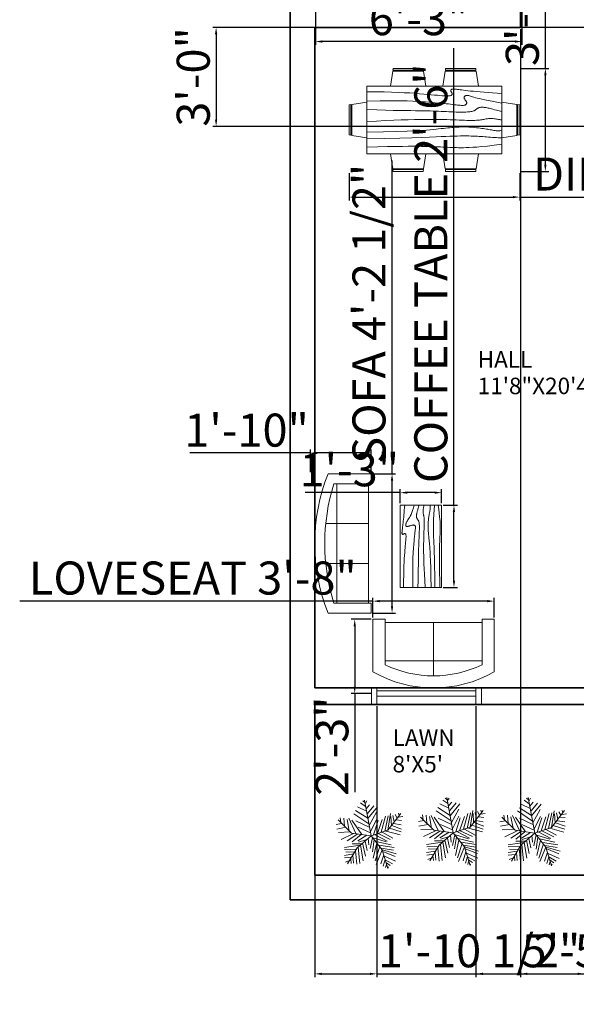
# Model space of a CAD drawing. Units: inches. Extents: x 2446 to 3341, y 462 to 1195.
# Tile 1 of 6: x 2446 to 2649, y 530 to 888. Entities that reach past the tile are written whole.
import ezdxf

# ---------------------------------------------------------------- set-up
doc = ezdxf.new("R2010")
doc.units = ezdxf.units.IN
for name, color, linetype, lineweight in [('A-ANNO-DIMS', 2, 'Continuous', 18), ('A-AREA-IDEN', 7, 'Continuous', 18), ('A-FURN', 8, 'Continuous', 18), ('A-GLAZ', 4, 'Continuous', 18), ('A-WALL', 7, 'Continuous', 35), ('C-PROP', 7, 'Continuous', 35), ('L-PLNT', 3, 'Continuous', 18)]:
    doc.layers.add(name, color=color, linetype=linetype, lineweight=lineweight)
doc.styles.get("Standard").update_dxf_attribs({"font": 'arial.ttf'})
doc.dimstyles.new('ISO-25', dxfattribs={"dimtxt": 12, "dimasz": 2.5, "dimexe": 1.25, "dimexo": 0.625, "dimtad": 1, "dimdec": 1, "dimlunit": 3, "dimtxsty": 'Standard', "dimcen": 2.5, "dimadec": 0, "dimazin": 0, "dimtfac": 1, "dimtdec": 1, "dimtmove": 0, "dimatfit": 3, "dimfxl": 1, "dimarcsym": 0})

# ---------------------------------------------------------------- blocks, each defined once
blk = doc.blocks.new('Sofa - Roundback 7 ft.')
for p, q in [((-36.000027, -34), (-36.000027, -11.4696)), ((-12.00002, -32.4421), (-12.00003, -6.5971)), ((11.99997, -32.4421), (11.99998, -6.5971)), ((35.99998, -34), (35.99998, -11.4696)), ((-35.999844, -13.3819), (35.9998, -13.3819)), ((-36.000027, -32.4421), (35.99998, -32.4421))]:
    blk.add_line(p, q)
for points in [[(-36.000027, -34), (-42.000027, -34), (-42.000027, -8)], [(41.99998, -8), (41.99998, -34), (35.99998, -34)]]:
    blk.add_lwpolyline(points)
for centre, radius, start, end in [((0, -114.25), 114.25, 68.43141, 111.5686), ((-0.00001, -127.1968), 121.1968, 72.72033, 107.2797)]:
    blk.add_arc(centre, radius, start, end)
blk = doc.blocks.new('Dining Set - 36 x 72 in.')
for p, q in [((-22, 27.5), (-22.1562, 26.50042)), ((-5.8416, 26.5), (-22.1534, 26.5)), ((-22, 27.5), (-6, 27.5)), ((-5.8437, 26.49966), (-6, 27.5)), ((6, 27.5), (5.8438, 26.50042)), ((22.1584, 26.5), (5.8466, 26.5)), ((6, 27.5), (22, 27.5)), ((22.1563, 26.49966), (22, 27.5)), ((-22.2343, 26.00059), (-23.4847, 17.99762)), ((-22.2304, 26), (-5.7608, 26)), ((-4.5152, 17.99762), (-5.7655, 25.99926)), ((5.7657, 26.00059), (4.5153, 17.99762)), ((5.7696, 26), (22.2392, 26)), ((23.4848, 17.99762), (22.2345, 25.99926)), ((36, 18), (-36, 18)), ((-36, 18), (-36, -18)), ((36, -18), (36, 18)), ((-45.5, 8), (-44.5004, 8.15617)), ((-45.5, 8), (-45.5, -8)), ((-44.5, -8.15843), (-44.5, 8.15338)), ((-44.0006, 8.23428), (-35.9976, 9.48474)), ((-44, 8.23041), (-44, -8.23915)), ((44.0006, 8.23428), (35.9976, 9.48474)), ((44, 8.23041), (44, -8.23915)), ((44.5, -8.15843), (44.5, 8.15338)), ((45.5, 8), (44.5005, 8.15617)), ((45.5, 8), (45.5, -8)), ((-44.4997, -8.15631), (-45.5, -8)), ((-35.9976, -9.48476), (-43.9993, -8.2345)), ((35.9976, -9.48476), (43.9993, -8.2345)), ((44.4997, -8.15631), (45.5, -8)), ((-36, -18), (36, -18)), ((-22.2343, -26.0006), (-23.4847, -17.99762)), ((-4.5152, -17.99762), (-5.7655, -25.99928)), ((5.7657, -26.0006), (4.5153, -17.99762)), ((23.4848, -17.99762), (22.2345, -25.99928)), ((-22.2304, -26), (-5.7608, -26)), ((5.7696, -26), (22.2392, -26)), ((-22, -27.5), (-22.1562, -26.50044)), ((-5.8416, -26.5), (-22.1534, -26.5)), ((-22, -27.5), (-6, -27.5)), ((-5.8437, -26.49967), (-6, -27.5)), ((6, -27.5), (5.8438, -26.50044)), ((22.1584, -26.5), (5.8466, -26.5)), ((6, -27.5), (22, -27.5)), ((22.1563, -26.49967), (22, -27.5))]:
    blk.add_line(p, q)
for points in [[(-36, 15), (-31.1772, 14.97754), (-26.8079, 14.91406), (-22.8538, 14.81543), (-19.276, 14.6875), (-16.0362, 14.53613), (-13.0957, 14.36718), (-10.4159, 14.18652), (-7.9583, 14), (-5.6904, 13.81315), (-3.6035, 13.63021), (-1.6954, 13.45508), (0.0365, 13.29166), (1.5945, 13.14388), (2.9811, 13.01562), (4.1988, 12.9108), (5.25, 12.83333), (6.1393, 12.78613), (6.8802, 12.76823), (7.4883, 12.77767), (7.9792, 12.8125), (8.3685, 12.87077), (8.6719, 12.95052), (8.9049, 13.0498), (9.0833, 13.16666), (9.2205, 13.29899), (9.3216, 13.44401), (9.3895, 13.59879), (9.4271, 13.76041), (9.4373, 13.92594), (9.4232, 14.09245), (9.3875, 14.257), (9.3333, 14.41666), (9.2638, 14.56917), (9.1836, 14.71484), (9.0975, 14.85465), (9.0104, 14.98958), (8.9272, 15.1206), (8.8529, 15.2487), (8.7922, 15.37483), (8.75, 15.5), (8.7305, 15.62467), (8.7344, 15.74739), (8.7617, 15.86621), (8.8125, 15.97916), (8.8867, 16.08431), (8.9844, 16.17968), (9.1055, 16.26334), (9.25, 16.33333), (9.4189, 16.38802), (9.6172, 16.42708), (9.8506, 16.45052), (10.125, 16.45833), (10.4463, 16.45052), (10.8203, 16.42708), (11.2529, 16.38802), (11.75, 16.33333), (12.3184, 16.26318), (12.9694, 16.17838), (13.7151, 16.07991), (14.5677, 15.96875), (15.5395, 15.84586), (16.6426, 15.71224), (17.8893, 15.56884), (19.2917, 15.41666), (20.859, 15.25667), (22.5879, 15.08984), (24.4721, 14.91715), (26.5052, 14.73958), (28.6809, 14.5581), (30.9929, 14.3737), (33.4347, 14.18733), (36, 14)], [(-36, 10), (-28.9766, 10.14274), (-23.1725, 10.20442), (-18.4241, 10.19775), (-14.5677, 10.13541), (-11.4399, 10.03011), (-8.877, 9.89453), (-6.7154, 9.74137), (-4.7917, 9.58333), (-2.9698, 9.43082), (-1.2246, 9.28515), (0.4415, 9.14534), (2.026, 9.01041), (3.5266, 8.87939), (4.9408, 8.7513), (6.266, 8.62516), (7.5, 8.5), (8.6411, 8.37549), (9.6914, 8.2539), (10.6538, 8.13818), (11.5312, 8.03125), (12.3267, 7.93603), (13.043, 7.85547), (13.6831, 7.79248), (14.25, 7.75), (14.7471, 7.7303), (15.1797, 7.73307), (15.5537, 7.75732), (15.875, 7.80208), (16.1494, 7.86637), (16.3828, 7.94922), (16.5811, 8.04964), (16.75, 8.16666), (16.8944, 8.29915), (17.0143, 8.44531), (17.1089, 8.60319), (17.1771, 8.77083), (17.218, 8.94629), (17.2305, 9.1276), (17.2137, 9.31282), (17.1667, 9.5), (17.0895, 9.6875), (16.987, 9.875), (16.8649, 10.0625), (16.7292, 10.25), (16.5856, 10.4375), (16.4401, 10.625), (16.2985, 10.8125), (16.1667, 11), (16.05, 11.18733), (15.9518, 11.3737), (15.8752, 11.5581), (15.8229, 11.73958), (15.798, 11.91715), (15.8034, 12.08984), (15.842, 12.25667), (15.9167, 12.41666), (16.0295, 12.56836), (16.1784, 12.70833), (16.3605, 12.83268), (16.5729, 12.9375), (16.8127, 13.01888), (17.0768, 13.07291), (17.3625, 13.0957), (17.6667, 13.08333), (17.9894, 13.03312), (18.3418, 12.94726), (18.7382, 12.82918), (19.1927, 12.68229), (19.7195, 12.51001), (20.3327, 12.31575), (21.0465, 12.10294), (21.875, 11.875), (22.8357, 11.63354), (23.959, 11.37304), (25.2786, 11.08618), (26.8282, 10.76562), (28.6414, 10.40405), (30.752, 9.99414), (33.1936, 9.52856), (36, 9)], [(-36, 5.5), (-30.7157, 5.3348), (-26.069, 5.20963), (-21.9946, 5.11767), (-18.4271, 5.05208), (-15.3009, 5.00602), (-12.5508, 4.97265), (-10.1112, 4.94515), (-7.9167, 4.91666), (-5.909, 4.88167), (-4.0586, 4.83984), (-2.3429, 4.79215), (-0.7396, 4.73958), (0.7739, 4.6831), (2.22, 4.6237), (3.6213, 4.56233), (5, 4.5), (6.373, 4.43782), (7.7344, 4.3776), (9.0723, 4.32129), (10.375, 4.27083), (11.6309, 4.22819), (12.8281, 4.19531), (13.9551, 4.17415), (15, 4.16666), (15.954, 4.17448), (16.819, 4.19791), (17.6001, 4.23698), (18.3021, 4.29166), (18.9299, 4.36198), (19.4883, 4.44791), (19.9823, 4.54948), (20.4167, 4.66666), (20.7969, 4.79899), (21.1302, 4.94401), (21.4245, 5.09879), (21.6875, 5.26041), (21.9271, 5.42594), (22.1511, 5.59245), (22.3672, 5.757), (22.5834, 5.91666), (22.8065, 6.06868), (23.0404, 6.21093), (23.2879, 6.34147), (23.5521, 6.45833), (23.8358, 6.55957), (24.142, 6.64323), (24.4735, 6.70735), (24.8334, 6.75), (25.2235, 6.76969), (25.642, 6.76692), (26.0858, 6.74267), (26.5521, 6.69791), (27.0379, 6.63362), (27.5404, 6.55078), (28.0565, 6.45036), (28.5834, 6.33333), (29.1242, 6.19987), (29.7071, 6.04687), (30.3661, 5.87044), (31.1354, 5.66666), (32.0493, 5.43164), (33.142, 5.16146), (34.4475, 4.85221), (36, 4.5)], [(-36, -1), (-30.7915, -0.6591), (-26.0195, -0.38216), (-21.6519, -0.16284), (-17.6563, 0.00521), (-14.0005, 0.12833), (-10.6523, 0.21289), (-7.5796, 0.26522), (-4.75, 0.29166), (-2.134, 0.29793), (0.2878, 0.28711), (2.5317, 0.26163), (4.6146, 0.22396), (6.5529, 0.17651), (8.3633, 0.12174), (10.0623, 0.06209), (11.6667, 0), (13.1899, -0.06201), (14.6341, -0.1211), (15.9982, -0.17432), (17.2813, -0.21875), (18.4823, -0.25147), (19.6003, -0.26953), (20.6343, -0.27002), (21.5834, -0.25), (22.4481, -0.20768), (23.2357, -0.14584), (23.9549, -0.06836), (24.6146, 0.02083), (25.2235, 0.11784), (25.7904, 0.21875), (26.3241, 0.31966), (26.8334, 0.41666), (27.3265, 0.50618), (27.8099, 0.58593), (28.2894, 0.65397), (28.7709, 0.70833), (29.2601, 0.74707), (29.763, 0.76823), (30.2855, 0.76985), (30.8334, 0.75), (31.4088, 0.70784), (31.9994, 0.64713), (32.589, 0.57275), (33.1615, 0.48958), (33.7008, 0.4025), (34.1908, 0.3164), (34.6153, 0.23616), (34.9584, 0.16666), (35.2099, 0.11165), (35.3848, 0.07031), (35.504, 0.04069), (35.5886, 0.02083), (35.6594, 0.00879), (35.7377, 0.0026), (35.8442, 0.00032), (36, 0)], [(-36, -6.5), (-27.1843, -6.31267), (-20.084, -6.1263), (-14.469, -5.9419), (-10.1094, -5.76042), (-6.7752, -5.58285), (-4.2363, -5.41016), (-2.2629, -5.24333), (-0.625, -5.08334), (0.8708, -4.93099), (2.2715, -4.78646), (3.5872, -4.64974), (4.8281, -4.52084), (6.0046, -4.39974), (7.127, -4.28646), (8.2053, -4.18099), (9.25, -4.08334), (10.2705, -3.99382), (11.2734, -3.91407), (12.2647, -3.84603), (13.25, -3.79167), (14.2354, -3.75293), (15.2266, -3.73177), (16.2295, -3.73015), (17.25, -3.75), (18.2912, -3.79248), (19.3451, -3.85547), (20.4009, -3.93604), (21.4479, -4.03125), (22.4754, -4.13819), (23.4727, -4.25391), (24.4289, -4.37549), (25.3334, -4.5), (26.1785, -4.62492), (26.9694, -4.74935), (27.7145, -4.87281), (28.4219, -4.99479), (29.1, -5.11483), (29.7572, -5.23242), (30.4016, -5.34709), (31.0417, -5.45834), (31.6837, -5.56437), (32.3262, -5.65821), (32.9658, -5.73153), (33.599, -5.77604), (34.2224, -5.78345), (34.8327, -5.74545), (35.4264, -5.65373), (36, -5.5)], [(-36, -10), (-26.4022, -9.81299), (-18.4675, -9.62891), (-11.9839, -9.45069), (-6.7396, -9.28125), (-2.5226, -9.12354), (0.8789, -8.98047), (3.6769, -8.85498), (6.0833, -8.75), (8.2767, -8.66765), (10.3021, -8.60677), (12.1712, -8.56543), (13.8958, -8.54167), (15.4876, -8.53353), (16.9583, -8.53907), (18.3197, -8.55632), (19.5834, -8.58334), (20.7616, -8.61841), (21.8685, -8.66081), (22.9188, -8.71004), (23.9271, -8.76563), (24.9081, -8.82707), (25.8763, -8.89388), (26.8465, -8.96558), (27.8334, -9.04167), (28.8474, -9.12118), (29.8828, -9.20117), (30.93, -9.27824), (31.9792, -9.34896), (33.0205, -9.40991), (34.0443, -9.45768), (35.0407, -9.48885), (36, -9.5)], [(-36, -14.5), (-30.0881, -14.33513), (-25.0332, -14.21224), (-20.7312, -14.12647), (-17.0781, -14.07292), (-13.97, -14.04671), (-11.3027, -14.04297), (-8.9724, -14.05681), (-6.875, -14.08334), (-4.9224, -14.11833), (-3.0905, -14.16016), (-1.3709, -14.20785), (0.2448, -14.26042), (1.7647, -14.3169), (3.1973, -14.3763), (4.5507, -14.43767), (5.8333, -14.5), (7.0554, -14.5621), (8.235, -14.62175), (9.3922, -14.67652), (10.5469, -14.72396), (11.7192, -14.76164), (12.929, -14.78711), (14.1965, -14.79794), (15.5417, -14.79167), (16.9933, -14.76424), (18.6152, -14.70508), (20.4804, -14.60197), (22.6615, -14.44271), (25.2312, -14.21509), (28.2624, -13.9069), (31.8277, -13.50594), (36, -13)]]:
    blk.add_lwpolyline(points)
blk = doc.blocks.new('Table - Rectangular Woodgrain 60 x 30 in.')
for p, q in [((0, 0), (0, -30)), ((60, 0), (0, 0)), ((60, -30), (60, 0)), ((0, -30), (60, -30))]:
    blk.add_line(p, q)
for points in [[(0, -2.4), (4.8155, -2.418), (9.0302, -2.4688), (12.709, -2.5477), (15.9167, -2.65), (18.7181, -2.7711), (21.1781, -2.9063), (23.3616, -3.0508), (25.3333, -3.2), (27.1477, -3.3495), (28.8172, -3.4958), (30.3437, -3.636), (31.7291, -3.7667), (32.9756, -3.8849), (34.0849, -3.9875), (35.059, -4.0714), (35.9, -4.1334), (36.6114, -4.1711), (37.2041, -4.1854), (37.6906, -4.1779), (38.0833, -4.15), (38.3948, -4.1034), (38.6375, -4.0396), (38.8239, -3.9602), (38.9666, -3.8667), (39.0764, -3.7608), (39.1573, -3.6448), (39.2116, -3.521), (39.2416, -3.3917), (39.2498, -3.2593), (39.2385, -3.1261), (39.21, -2.9944), (39.1666, -2.8667), (39.111, -2.7447), (39.0468, -2.6281), (38.978, -2.5163), (38.9083, -2.4083), (38.8418, -2.3035), (38.7823, -2.201), (38.7337, -2.1001), (38.7, -2), (38.6844, -1.9003), (38.6875, -1.8021), (38.7094, -1.707), (38.75, -1.6167), (38.8094, -1.5326), (38.8875, -1.4563), (38.9844, -1.3893), (39.1, -1.3333), (39.2351, -1.2896), (39.3937, -1.2583), (39.5804, -1.2396), (39.8, -1.2333), (40.057, -1.2396), (40.3562, -1.2583), (40.7023, -1.2896), (41.1, -1.3333), (41.5547, -1.3895), (42.0755, -1.4573), (42.6721, -1.5361), (43.3542, -1.625), (44.1316, -1.7233), (45.014, -1.8302), (46.0114, -1.9449), (47.1333, -2.0667), (48.3862, -2.1947), (49.7625, -2.3281), (51.2513, -2.4663), (52.8416, -2.6083), (54.5226, -2.7535), (56.2833, -2.9011), (58.1127, -3.0501), (60, -3.2)], [(0, -9.2), (6.5759, -9.0858), (11.9385, -9.0365), (16.2527, -9.0418), (19.6833, -9.0917), (22.3952, -9.1759), (24.5531, -9.2844), (26.322, -9.4069), (27.8666, -9.5333), (29.3241, -9.6553), (30.7203, -9.7719), (32.0532, -9.8837), (33.3208, -9.9917), (34.5213, -10.0965), (35.6526, -10.199), (36.7128, -10.2999), (37.7, -10.4), (38.6129, -10.4996), (39.4531, -10.5969), (40.223, -10.6895), (40.925, -10.775), (41.5613, -10.8512), (42.1344, -10.9156), (42.6465, -10.966), (43.1, -11), (43.4976, -11.0158), (43.8437, -11.0136), (44.143, -10.9942), (44.4, -10.9583), (44.6195, -10.9069), (44.8062, -10.8406), (44.9648, -10.7603), (45.1, -10.6667), (45.2155, -10.5598), (45.3114, -10.4365), (45.3871, -10.2929), (45.4416, -10.125), (45.4743, -9.929), (45.4844, -9.7011), (45.4709, -9.4371), (45.4333, -9.1333), (45.3716, -8.7883), (45.2896, -8.4104), (45.1919, -8.0107), (45.0833, -7.6), (44.9685, -7.1893), (44.8521, -6.7896), (44.7388, -6.4117), (44.6333, -6.0667), (44.54, -5.7628), (44.4614, -5.4979), (44.4001, -5.2675), (44.3583, -5.0667), (44.3384, -4.8909), (44.3427, -4.7354), (44.3736, -4.5956), (44.4333, -4.4667), (44.5236, -4.3453), (44.6427, -4.2333), (44.7884, -4.1339), (44.9583, -4.05), (45.1501, -3.9849), (45.3614, -3.9417), (45.59, -3.9234), (45.8333, -3.9333), (46.0915, -3.9749), (46.3734, -4.0531), (46.6906, -4.1736), (47.0542, -4.3417), (47.4756, -4.5629), (47.9661, -4.8427), (48.5372, -5.1866), (49.2, -5.6), (49.9676, -6.0844), (50.8594, -6.625), (51.8965, -7.2031), (53.1, -7.8), (54.491, -8.3969), (56.0906, -8.975), (57.9199, -9.5156), (60, -10)], [(0, -12.8), (5.1847, -12.9322), (9.6213, -13.0323), (13.3963, -13.1059), (16.5958, -13.1583), (19.3063, -13.1952), (21.614, -13.2219), (23.6054, -13.2439), (25.3666, -13.2667), (26.9728, -13.2947), (28.4531, -13.3281), (29.8256, -13.3663), (31.1083, -13.4083), (32.3191, -13.4535), (33.476, -13.501), (34.597, -13.5501), (35.7, -13.6), (36.7984, -13.6497), (37.8875, -13.6979), (38.9578, -13.743), (40, -13.7833), (41.0047, -13.8174), (41.9625, -13.8438), (42.864, -13.8607), (43.7, -13.8667), (44.4631, -13.8604), (45.1552, -13.8417), (45.7801, -13.8104), (46.3416, -13.7667), (46.8439, -13.7104), (47.2906, -13.6417), (47.6858, -13.5604), (48.0333, -13.4667), (48.3375, -13.3608), (48.6042, -13.2448), (48.8396, -13.121), (49.05, -12.9917), (49.2417, -12.8593), (49.4208, -12.7261), (49.5937, -12.5944), (49.7667, -12.4667), (49.9452, -12.3451), (50.1323, -12.2313), (50.3303, -12.1268), (50.5416, -12.0333), (50.7686, -11.9524), (51.0135, -11.8854), (51.2788, -11.8341), (51.5666, -11.8), (51.8785, -11.7843), (52.2116, -11.7865), (52.562, -11.8059), (52.926, -11.8417), (53.2998, -11.8931), (53.6795, -11.9594), (54.0614, -12.0397), (54.4416, -12.1333), (54.8223, -12.2401), (55.2293, -12.3625), (55.6942, -12.5037), (56.2489, -12.6667), (56.9251, -12.8547), (57.7545, -13.0708), (58.7689, -13.3182), (60, -13.6)], [(0, -18), (5.124, -17.7273), (9.6609, -17.5057), (13.6705, -17.3303), (17.2125, -17.1958), (20.3467, -17.0973), (23.1328, -17.0297), (25.6307, -16.9878), (27.9, -16.9667), (29.9928, -16.9617), (31.9302, -16.9703), (33.7254, -16.9907), (35.3917, -17.0208), (36.9423, -17.0588), (38.3906, -17.1026), (39.7499, -17.1503), (41.0333, -17.2), (42.2519, -17.2496), (43.4073, -17.2969), (44.4986, -17.3395), (45.525, -17.375), (46.4858, -17.4012), (47.3802, -17.4156), (48.2074, -17.416), (48.9667, -17.4), (49.6583, -17.3662), (50.2872, -17.3167), (50.8595, -17.2547), (51.3812, -17.1833), (51.8584, -17.1057), (52.2971, -17.025), (52.7034, -16.9443), (53.0833, -16.8667), (53.443, -16.7951), (53.789, -16.7313), (54.128, -16.6768), (54.4666, -16.6334), (54.8115, -16.6024), (55.1693, -16.5854), (55.5465, -16.5841), (55.95, -16.6), (56.3828, -16.6337), (56.8346, -16.6823), (57.2915, -16.7418), (57.7396, -16.8084), (58.165, -16.878), (58.5539, -16.9469), (58.8924, -17.0111), (59.1666, -17.0667), (59.3679, -17.1107), (59.5078, -17.1438), (59.6032, -17.1675), (59.6708, -17.1833), (59.7275, -17.193), (59.7901, -17.1979), (59.8753, -17.1998), (60, -17.2)], [(0, -22.4), (8.0098, -22.2501), (14.4094, -22.1011), (19.4168, -21.9535), (23.25, -21.8083), (26.1269, -21.6663), (28.2656, -21.5281), (29.884, -21.3947), (31.2, -21.2667), (32.3967, -21.1448), (33.5172, -21.0292), (34.5697, -20.9198), (35.5625, -20.8167), (36.5037, -20.7198), (37.4015, -20.6292), (38.2642, -20.5448), (39.1, -20.4667), (39.9164, -20.3951), (40.7187, -20.3313), (41.5117, -20.2768), (42.3, -20.2333), (43.0883, -20.2024), (43.8812, -20.1854), (44.6836, -20.1841), (45.5, -20.2), (46.3328, -20.234), (47.1747, -20.2844), (48.0163, -20.3488), (48.8479, -20.425), (49.66, -20.5106), (50.4429, -20.6031), (51.1872, -20.7004), (51.8833, -20.8), (52.5246, -20.8999), (53.1166, -20.9995), (53.6681, -21.0983), (54.1875, -21.1958), (54.6834, -21.2919), (55.1646, -21.3859), (55.6394, -21.4777), (56.1167, -21.5667), (56.6028, -21.6515), (57.0961, -21.7266), (57.5929, -21.7852), (58.0896, -21.8208), (58.5823, -21.8268), (59.0674, -21.7964), (59.5412, -21.723), (60, -21.6)], [(0, -25.2), (8.6355, -25.0504), (15.7026, -24.9031), (21.4049, -24.7606), (25.9458, -24.625), (29.529, -24.4988), (32.3578, -24.3844), (34.6359, -24.284), (36.5667, -24.2), (38.3213, -24.1341), (39.9417, -24.0854), (41.437, -24.0523), (42.8167, -24.0333), (44.0901, -24.0268), (45.2667, -24.0313), (46.3557, -24.0451), (47.3667, -24.0667), (48.309, -24.0947), (49.1928, -24.1287), (50.0284, -24.168), (50.826, -24.2125), (51.5959, -24.2617), (52.3483, -24.3151), (53.0935, -24.3725), (53.8417, -24.4334), (54.6009, -24.497), (55.3699, -24.561), (56.1454, -24.6226), (56.9239, -24.6792), (57.7021, -24.7279), (58.4764, -24.7662), (59.2435, -24.7911), (60, -24.8)], [(0, -28.8), (5.6867, -28.6681), (10.45, -28.5698), (14.407, -28.5012), (17.675, -28.4584), (20.3711, -28.4374), (22.6125, -28.4344), (24.5164, -28.4455), (26.2, -28.4667), (27.762, -28.4947), (29.2276, -28.5281), (30.6033, -28.5663), (31.8958, -28.6084), (33.1118, -28.6535), (34.2578, -28.7011), (35.3405, -28.7501), (36.3666, -28.8), (37.3443, -28.8497), (38.288, -28.8974), (39.2137, -28.9412), (40.1375, -28.9792), (41.0753, -29.0093), (42.0432, -29.0297), (43.0572, -29.0384), (44.1333, -29.0333), (45.2936, -29.0114), (46.5843, -28.9641), (48.0579, -28.8816), (49.7666, -28.7542), (51.7629, -28.5721), (54.0989, -28.3255), (56.8272, -28.0048), (60, -27.6)]]:
    blk.add_lwpolyline(points)
blk = doc.blocks.new('Sofa - Roundback Loveseat 5 ft.')
for p, q in [((0, -32.44198), (0, -5.99998)), ((-24, -33.99998), (-24, -11.46958)), ((-23.9998, -13.38178), (23.99986, -13.38178)), ((24.00004, -33.99998), (24.00004, -11.46958)), ((-24, -32.44198), (24.00004, -32.44198))]:
    blk.add_line(p, q)
for points in [[(-24, -33.99998), (-30, -33.99998), (-30, -7.99998)], [(30.00004, -7.99998), (30.00004, -33.99998), (24.00004, -33.99998)]]:
    blk.add_lwpolyline(points)
for centre, radius, start, end in [((0, -60.24998), 60.24998, 60.13715, 119.8628), ((0, -61.38438), 55.38444, 64.32083, 115.6792)]:
    blk.add_arc(centre, radius, start, end)
blk = doc.blocks.new('*U16')
for p, q in [((-8.737, 47.138), (-17.069, 52.711)), ((-10.186, 53.64), (-13.084, 55.962)), ((0, 0), (-10.5, 57)), ((-9.099, 51.782), (-6.563, 55.962)), ((-7.65, 43.423), (-2.578, 49.46)), ((-5.839, 35.992), (4.667, 48.067)), ((-3.665, 19.273), (-27.574, 35.527)), ((-5.114, 28.097), (-24.676, 40.636)), ((-7.288, 39.707), (-21.778, 46.673)), ((-5.114, 27.632), (10.463, 46.673)), ((-2.941, 16.486), (8.652, 37.85)), ((22.055, 7.198), (27.489, 32.277)), ((27, 9), (48, 36)), ((27.127, 9.056), (31.112, 35.992)), ((35.096, 32.741), (37.27, 22.524)), ((38.719, 34.134), (41.979, 28.561)), ((44.153, 36.456), (45.239, 32.741)), ((-47.498, 19.737), (-55.83, 18.344)), ((-31.5, 4.5), (-52.5, 25.5)), ((-48.585, 21.131), (-49.309, 29.026)), ((-43.513, 28.561), (-42.427, 15.558)), ((-38.442, 26.239), (-34.819, 7.663)), ((-35.544, 28.097), (-24.314, 3.947)), ((-14.533, 2.09), (-30.834, 25.31)), ((-24.314, 23.917), (-2.941, 13.7)), ((-1.129, 6.734), (9.014, 26.704)), ((3.942, 1.625), (11.187, 24.381)), ((10.101, 3.483), (17.708, 26.239)), ((16.259, 5.805), (23.142, 31.348)), ((31.836, 30.883), (32.561, 16.486)), ((33.285, 16.486), (48.862, 10.913)), ((36.183, 19.737), (48.137, 17.88)), ((40.53, 25.775), (48.862, 24.846)), ((43.791, 29.954), (51.036, 30.883)), ((-40.615, 13.7), (-55.105, 10.913)), ((-33.37, 6.269), (-52.207, 5.34)), ((-28.299, 3.483), (-47.86, -5.805)), ((-21.416, 3.018), (-38.079, -8.128)), ((0, 0), (-31.5, 4.5)), ((-15.982, 2.09), (-30.11, -9.521)), ((0, 0), (-22.5, -19.5)), ((-6.563, 1.161), (-21.416, -8.128)), ((-20.691, 13.7), (-1.129, 4.876)), ((0, 0), (27, 9)), ((0, 0), (18, -22.5)), ((6.478, 1.625), (26.04, -8.592)), ((11.187, 3.483), (30.749, -5.805)), ((18.07, 5.805), (35.096, -3.483)), ((24.229, 7.663), (46.688, 1.625)), ((29.662, 12.307), (48.137, 6.269)), ((-17.431, -15.094), (-42.789, -18.809)), ((-15.257, -12.772), (-30.11, -12.772)), ((-6.563, -5.805), (-19.967, -9.985)), ((-17.069, -15.094), (-12.721, -40.172)), ((-13.446, -11.378), (-8.737, -32.741)), ((-9.461, -8.592), (-6.201, -23.453)), ((-4.752, -3.483), (-3.665, -14.629)), ((2.493, -3.019), (-1.491, -20.202)), ((1.769, -2.555), (24.229, -9.521)), ((5.029, -6.27), (2.131, -25.775)), ((9.014, -11.378), (3.58, -35.992)), ((7.565, -9.056), (32.198, -14.629)), ((12.274, -15.094), (36.907, -18.809)), ((-28.299, -29.026), (-42.789, -31.348)), ((-24.314, -21.596), (-42.427, -22.06)), ((-26.849, -26.24), (-40.253, -25.775)), ((-22.5, -19.5), (-37.5, -45)), ((-29.023, -30.884), (-27.936, -43.887)), ((-25.038, -23.918), (-22.865, -45.281)), ((-20.691, -18.345), (-17.793, -44.352)), ((14.085, -16.951), (6.478, -40.172)), ((18.07, -22.524), (8.289, -45.745)), ((20.244, -30.419), (15.897, -44.816)), ((16.259, -19.738), (36.183, -22.989)), ((18, -22.5), (27, -52.5)), ((18.433, -22.524), (40.53, -29.026)), ((19.157, -25.311), (38.719, -33.206)), ((-30.834, -34.135), (-42.427, -35.528)), ((-34.457, -39.708), (-40.978, -42.494)), ((-32.646, -36.921), (-31.921, -44.352)), ((22.78, -37.85), (19.519, -48.532)), ((21.331, -32.741), (39.081, -40.636)), ((22.78, -38.314), (34.372, -44.816)), ((24.591, -45.745), (23.142, -50.854)), ((24.591, -43.423), (30.749, -47.603)), ((26.764, -49.925), (28.213, -50.854))]:
    blk.add_line(p, q)
blk = doc.blocks.new('WIN-36IN')
for p, q in [((0, 6), (0, 0)), ((0, 5), (36, 5)), ((36, 0), (36, 6)), ((0, 3), (36, 3))]:
    blk.add_line(p, q)
blk = doc.blocks.new('*D51')
at = {"layer": 'A-ANNO-DIMS', "color": 0, "lineweight": -2, "transparency": 16777216}
for p, q in [((2581.67, 722.76), (2581.67, 836.62)), ((2574.71, 722.76), (2582.92, 722.76)), ((2581.67, 674.69), (2581.67, 720.26)), ((2574.71, 672.19), (2582.92, 672.19))]:
    blk.add_line(p, q, dxfattribs=at)
at = {"layer": 'A-ANNO-DIMS', "color": 0, "transparency": 16777216}
for points in [[(2581.25, 720.26), (2582.09, 720.26), (2581.67, 722.76)], [(2581.25, 674.69), (2582.09, 674.69), (2581.67, 672.19)]]:
    blk.add_solid(points, dxfattribs=at)
at = {"layer": 'Defpoints', "color": 0, "transparency": 16777216}
for p in [(2574.08, 722.76), (2581.67, 722.76), (2574.08, 672.19)]:
    blk.add_point(p, dxfattribs=at)
at = {"layer": 'A-ANNO-DIMS', "color": 0, "transparency": 16777216, "insert": (2574.84, 780.94), "char_height": 12, "attachment_point": 5, "rotation": 90}
blk.add_mtext('SOFA 4\'-2 1/2"', dxfattribs=at)
blk = doc.blocks.new('*D52')
at = {"layer": 'A-ANNO-DIMS', "color": 0, "lineweight": -2, "transparency": 16777216}
for p, q in [((2552.01, 730.35), (2508.17, 730.35)), ((2552.01, 723.39), (2552.01, 731.6)), ((2571.58, 730.35), (2554.51, 730.35)), ((2574.08, 723.39), (2574.08, 731.6))]:
    blk.add_line(p, q, dxfattribs=at)
at = {"layer": 'A-ANNO-DIMS', "color": 0, "transparency": 16777216}
for points in [[(2554.51, 730.77), (2554.51, 729.93), (2552.01, 730.35)], [(2571.58, 730.77), (2571.58, 729.93), (2574.08, 730.35)]]:
    blk.add_solid(points, dxfattribs=at)
at = {"layer": 'Defpoints', "color": 0, "transparency": 16777216}
for p in [(2552.01, 730.35), (2552.01, 722.76), (2574.08, 722.76)]:
    blk.add_point(p, dxfattribs=at)
at = {"layer": 'A-ANNO-DIMS', "color": 0, "transparency": 16777216, "insert": (2528.84, 737.1), "char_height": 12, "attachment_point": 5}
blk.add_mtext('1\'-10"', dxfattribs=at)
blk = doc.blocks.new('*D53')
at = {"layer": 'A-ANNO-DIMS', "color": 0, "lineweight": -2, "transparency": 16777216}
for p, q in [((2566.04, 831.98), (2566.04, 822.05)), ((2628.06, 831.98), (2628.06, 822.05)), ((2568.54, 823.3), (2625.56, 823.3)), ((2628.06, 823.3), (2763.7, 823.3))]:
    blk.add_line(p, q, dxfattribs=at)
at = {"layer": 'A-ANNO-DIMS', "color": 0, "transparency": 16777216}
for points in [[(2568.54, 823.72), (2568.54, 822.89), (2566.04, 823.3)], [(2625.56, 823.72), (2625.56, 822.89), (2628.06, 823.3)]]:
    blk.add_solid(points, dxfattribs=at)
at = {"layer": 'Defpoints', "color": 0, "transparency": 16777216}
for p in [(2566.04, 832.6), (2628.06, 832.6), (2628.06, 823.3)]:
    blk.add_point(p, dxfattribs=at)
at = {"layer": 'A-ANNO-DIMS', "color": 0, "transparency": 16777216, "insert": (2697.13, 830.13), "char_height": 12, "attachment_point": 5}
blk.add_mtext('DINING SET 5\'-2"', dxfattribs=at)
blk = doc.blocks.new('*D54')
at = {"layer": 'A-ANNO-DIMS', "color": 0, "lineweight": -2, "transparency": 16777216}
for p, q in [((2637.36, 870.08), (2637.36, 933.69)), ((2628.68, 870.08), (2638.61, 870.08)), ((2637.36, 835.1), (2637.36, 867.58)), ((2628.68, 832.6), (2638.61, 832.6))]:
    blk.add_line(p, q, dxfattribs=at)
at = {"layer": 'A-ANNO-DIMS', "color": 0, "transparency": 16777216}
for points in [[(2636.94, 867.58), (2637.77, 867.58), (2637.36, 870.08)], [(2636.94, 835.1), (2637.77, 835.1), (2637.36, 832.6)]]:
    blk.add_solid(points, dxfattribs=at)
at = {"layer": 'Defpoints', "color": 0, "transparency": 16777216}
for p in [(2628.06, 870.08), (2637.36, 870.08), (2628.06, 832.6)]:
    blk.add_point(p, dxfattribs=at)
at = {"layer": 'A-ANNO-DIMS', "color": 0, "transparency": 16777216, "insert": (2630.52, 903.14), "char_height": 12, "attachment_point": 5, "rotation": 90}
blk.add_mtext('3\'-1 1/2"', dxfattribs=at)
blk = doc.blocks.new('*D56')
at = {"layer": 'A-ANNO-DIMS', "color": 0, "lineweight": -2, "transparency": 16777216}
for p, q in [((2553.87, 891.87), (2553.87, 878.58)), ((2628.78, 891.87), (2628.78, 878.58)), ((2626.28, 879.83), (2556.37, 879.83))]:
    blk.add_line(p, q, dxfattribs=at)
at = {"layer": 'A-ANNO-DIMS', "color": 0, "transparency": 16777216}
for points in [[(2556.37, 880.24), (2556.37, 879.41), (2553.87, 879.83)], [(2626.28, 880.24), (2626.28, 879.41), (2628.78, 879.83)]]:
    blk.add_solid(points, dxfattribs=at)
at = {"layer": 'Defpoints', "color": 0, "transparency": 16777216}
for p in [(2553.87, 892.5), (2628.78, 892.5), (2553.87, 879.83)]:
    blk.add_point(p, dxfattribs=at)
at = {"layer": 'A-ANNO-DIMS', "color": 0, "transparency": 16777216, "insert": (2591.32, 886.58), "char_height": 12, "attachment_point": 5}
blk.add_mtext('6\'-3"', dxfattribs=at)
blk = doc.blocks.new('*D57')
at = {"layer": 'A-ANNO-DIMS', "color": 0, "lineweight": -2, "transparency": 16777216}
for p, q in [((2604.16, 711.44), (2604.16, 877.37)), ((2600.28, 711.44), (2605.41, 711.44)), ((2604.16, 683.95), (2604.16, 708.94)), ((2600.28, 681.45), (2605.41, 681.45))]:
    blk.add_line(p, q, dxfattribs=at)
at = {"layer": 'A-ANNO-DIMS', "color": 0, "transparency": 16777216}
for points in [[(2603.74, 708.94), (2604.57, 708.94), (2604.16, 711.44)], [(2603.74, 683.95), (2604.57, 683.95), (2604.16, 681.45)]]:
    blk.add_solid(points, dxfattribs=at)
at = {"layer": 'Defpoints', "color": 0, "transparency": 16777216}
for p in [(2599.66, 711.44), (2604.16, 711.44), (2599.66, 681.45)]:
    blk.add_point(p, dxfattribs=at)
at = {"layer": 'A-ANNO-DIMS', "color": 0, "transparency": 16777216, "insert": (2597.32, 795.66), "char_height": 12, "attachment_point": 5, "rotation": 90}
blk.add_mtext('COFFEE TABLE 2\'-6"', dxfattribs=at)
blk = doc.blocks.new('*D58')
at = {"layer": 'A-ANNO-DIMS', "color": 0, "lineweight": -2, "transparency": 16777216}
for p, q in [((2584.66, 715.94), (2550.14, 715.94)), ((2584.66, 712.07), (2584.66, 717.19)), ((2597.16, 715.94), (2587.16, 715.94)), ((2599.66, 712.07), (2599.66, 717.19))]:
    blk.add_line(p, q, dxfattribs=at)
at = {"layer": 'A-ANNO-DIMS', "color": 0, "transparency": 16777216}
for points in [[(2587.16, 716.36), (2587.16, 715.53), (2584.66, 715.94)], [(2597.16, 716.36), (2597.16, 715.53), (2599.66, 715.94)]]:
    blk.add_solid(points, dxfattribs=at)
at = {"layer": 'Defpoints', "color": 0, "transparency": 16777216}
for p in [(2584.66, 715.94), (2584.66, 711.44), (2599.66, 711.44)]:
    blk.add_point(p, dxfattribs=at)
at = {"layer": 'A-ANNO-DIMS', "color": 0, "transparency": 16777216, "insert": (2566.15, 722.7), "char_height": 12, "attachment_point": 5}
blk.add_mtext('1\'-3"', dxfattribs=at)
blk = doc.blocks.new('*D59')
at = {"layer": 'A-ANNO-DIMS', "color": 0, "lineweight": -2, "transparency": 16777216}
for p, q in [((2574.71, 676.53), (2446.43, 676.53)), ((2574.71, 670.55), (2574.71, 677.78)), ((2616.25, 676.53), (2577.21, 676.53)), ((2618.75, 670.55), (2618.75, 677.78))]:
    blk.add_line(p, q, dxfattribs=at)
at = {"layer": 'A-ANNO-DIMS', "color": 0, "transparency": 16777216}
for points in [[(2577.21, 676.94), (2577.21, 676.11), (2574.71, 676.53)], [(2616.25, 676.94), (2616.25, 676.11), (2618.75, 676.53)]]:
    blk.add_solid(points, dxfattribs=at)
at = {"layer": 'Defpoints', "color": 0, "transparency": 16777216}
for p in [(2574.71, 676.53), (2574.71, 669.92), (2618.75, 669.92)]:
    blk.add_point(p, dxfattribs=at)
at = {"layer": 'A-ANNO-DIMS', "color": 0, "transparency": 16777216, "insert": (2509.32, 683.36), "char_height": 12, "attachment_point": 5}
blk.add_mtext('LOVESEAT 3\'-8"', dxfattribs=at)
blk = doc.blocks.new('*D60')
at = {"layer": 'A-ANNO-DIMS', "color": 0, "lineweight": -2, "transparency": 16777216}
for p, q in [((2574.09, 669.92), (2566.86, 669.92)), ((2568.11, 667.42), (2568.11, 645.51)), ((2574.09, 643.01), (2566.86, 643.01)), ((2568.11, 643.01), (2568.11, 607.16))]:
    blk.add_line(p, q, dxfattribs=at)
at = {"layer": 'A-ANNO-DIMS', "color": 0, "transparency": 16777216}
for points in [[(2567.69, 667.42), (2568.52, 667.42), (2568.11, 669.92)], [(2567.69, 645.51), (2568.52, 645.51), (2568.11, 643.01)]]:
    blk.add_solid(points, dxfattribs=at)
at = {"layer": 'Defpoints', "color": 0, "transparency": 16777216}
for p in [(2574.71, 669.92), (2568.11, 643.01), (2574.71, 643.01)]:
    blk.add_point(p, dxfattribs=at)
at = {"layer": 'A-ANNO-DIMS', "color": 0, "transparency": 16777216, "insert": (2561.35, 623.84), "char_height": 12, "attachment_point": 5, "rotation": 90}
blk.add_mtext('2\'-3"', dxfattribs=at)
blk = doc.blocks.new('*D63')
at = {"layer": 'A-ANNO-DIMS', "color": 0, "lineweight": -2, "transparency": 16777216}
for p, q in [((2700.99, 884.97), (2516.52, 884.97)), ((2517.77, 882.47), (2517.77, 851.47)), ((2700.99, 848.97), (2516.52, 848.97))]:
    blk.add_line(p, q, dxfattribs=at)
at = {"layer": 'A-ANNO-DIMS', "color": 0, "transparency": 16777216}
for points in [[(2517.35, 882.47), (2518.18, 882.47), (2517.77, 884.97)], [(2517.35, 851.47), (2518.18, 851.47), (2517.77, 848.97)]]:
    blk.add_solid(points, dxfattribs=at)
at = {"layer": 'Defpoints', "color": 0, "transparency": 16777216}
for p in [(2701.62, 884.97), (2517.77, 848.97), (2701.62, 848.97)]:
    blk.add_point(p, dxfattribs=at)
at = {"layer": 'A-ANNO-DIMS', "color": 0, "transparency": 16777216, "insert": (2511.01, 866.97), "char_height": 12, "attachment_point": 5, "rotation": 90}
blk.add_mtext('3\'-0"', dxfattribs=at)
blk = doc.blocks.new('*D71')
at = {"layer": 'A-ANNO-DIMS', "color": 0, "lineweight": -2, "transparency": 16777216}
for p, q in [((2553.62, 638.34), (2553.62, 539.87)), ((2576.15, 638.34), (2576.15, 539.87)), ((2556.12, 541.12), (2573.65, 541.12)), ((2576.15, 541.12), (2647.95, 541.12))]:
    blk.add_line(p, q, dxfattribs=at)
at = {"layer": 'A-ANNO-DIMS', "color": 0, "transparency": 16777216}
for points in [[(2556.12, 541.54), (2556.12, 540.7), (2553.62, 541.12)], [(2573.65, 541.54), (2573.65, 540.7), (2576.15, 541.12)]]:
    blk.add_solid(points, dxfattribs=at)
at = {"layer": 'Defpoints', "color": 0, "transparency": 16777216}
for p in [(2553.62, 638.97), (2576.15, 638.97), (2576.15, 541.12)]:
    blk.add_point(p, dxfattribs=at)
at = {"layer": 'A-ANNO-DIMS', "color": 0, "transparency": 16777216, "insert": (2613.3, 547.95), "char_height": 12, "attachment_point": 5}
blk.add_mtext('1\'-10 1/2"', dxfattribs=at)
blk = doc.blocks.new('*D72')
at = {"layer": 'A-ANNO-DIMS', "color": 0, "lineweight": -2, "transparency": 16777216}
for p, q in [((2612.15, 638.34), (2612.15, 539.87)), ((2651.62, 638.34), (2651.62, 539.87)), ((2614.65, 541.12), (2649.12, 541.12)), ((2651.62, 541.12), (2715.22, 541.12))]:
    blk.add_line(p, q, dxfattribs=at)
at = {"layer": 'A-ANNO-DIMS', "color": 0, "transparency": 16777216}
for points in [[(2614.65, 541.54), (2614.65, 540.7), (2612.15, 541.12)], [(2649.12, 541.54), (2649.12, 540.7), (2651.62, 541.12)]]:
    blk.add_solid(points, dxfattribs=at)
at = {"layer": 'Defpoints', "color": 0, "transparency": 16777216}
for p in [(2612.15, 638.97), (2651.62, 638.97), (2651.62, 541.12)]:
    blk.add_point(p, dxfattribs=at)
at = {"layer": 'A-ANNO-DIMS', "color": 0, "transparency": 16777216, "insert": (2684.67, 547.95), "char_height": 12, "attachment_point": 5}
blk.add_mtext('3\'-3 1/2"', dxfattribs=at)
blk = doc.blocks.new('*D74')
at = {"layer": 'A-ANNO-DIMS', "color": 0, "lineweight": -2, "transparency": 16777216}
for p, q in [((2628.27, 884.34), (2628.27, 539.87)), ((2693.62, 884.34), (2693.62, 539.87)), ((2630.77, 541.12), (2691.12, 541.12))]:
    blk.add_line(p, q, dxfattribs=at)
at = {"layer": 'A-ANNO-DIMS', "color": 0, "transparency": 16777216}
for points in [[(2630.77, 541.54), (2630.77, 540.7), (2628.27, 541.12)], [(2691.12, 541.54), (2691.12, 540.7), (2693.62, 541.12)]]:
    blk.add_solid(points, dxfattribs=at)
at = {"layer": 'Defpoints', "color": 0, "transparency": 16777216}
for p in [(2628.27, 884.97), (2693.62, 884.97), (2693.62, 541.12)]:
    blk.add_point(p, dxfattribs=at)
at = {"layer": 'A-ANNO-DIMS', "color": 0, "transparency": 16777216, "insert": (2660.94, 547.95), "char_height": 12, "attachment_point": 5}
blk.add_mtext('5\'-5 1/2"', dxfattribs=at)

msp = doc.modelspace()

# ---------------------------------------------------------------- linework, layer by layer
at = {"layer": 'A-GLAZ'}
for p, q in [((2574.15, 644.97), (2574.15, 638.97)), ((2614.15, 638.97), (2614.15, 644.97))]:
    msp.add_line(p, q, dxfattribs=at)
at = {"layer": 'A-WALL'}
for p, q in [((2628.27, 890.97), (2628.27, 884.97)), ((2553.62, 884.97), (2553.62, 644.97)), ((2628.27, 884.97), (2553.62, 884.97)), ((2651.62, 644.97), (2553.62, 644.97)), ((2553.62, 638.97), (2553.62, 576.97)), ((2651.62, 638.97), (2553.62, 638.97)), ((2553.62, 576.97), (2693.62, 576.97))]:
    msp.add_line(p, q, dxfattribs=at)
at = {"layer": 'C-PROP'}
msp.add_lwpolyline([(2544.62, 567.97), (2844.62, 567.97), (2844.62, 1047.97), (2544.62, 1047.97)], close=True, dxfattribs=at)

# ---------------------------------------------------------------- block references
at = {"layer": 'A-FURN', "xscale": 0.6814551436135577, "yscale": 0.6814551436135577, "zscale": 0.6814551436135577}
msp.add_blockref('Dining Set - 36 x 72 in.', (2597.05, 851.34), dxfattribs=at)
at = {"layer": 'A-FURN'}
for name, p, xscale, yscale, zscale, rotation in [('Sofa - Roundback 7 ft.', (2553.61, 697.48), 0.6020644949727707, 0.6020644949727707, 0.6020644949727707, 90), ('Table - Rectangular Woodgrain 60 x 30 in.', (2584.66, 681.45), 0.4998412302571817, 0.4998412302571817, 0.4998412302571817, 90), ('Sofa - Roundback Loveseat 5 ft.', (2596.73, 644.97), 0.7338992872016372, 0.7338992872016372, 0.7338992872016372, 180)]:
    msp.add_blockref(name, p, dxfattribs=dict(at, xscale=xscale, yscale=yscale, zscale=zscale, rotation=rotation))
at = {"layer": 'A-GLAZ'}
msp.add_blockref('WIN-36IN', (2576.15, 638.97), dxfattribs=at)
at = {"layer": 'L-PLNT', "xscale": 0.2264912736033225, "yscale": 0.2264912736033225, "zscale": 0.2264912736033225}
for p in [(2603.92, 592.32), (2633.49, 592.25), (2574.04, 591.26)]:
    msp.add_blockref('*U16', p, dxfattribs=at)

# ---------------------------------------------------------------- texts
at = {"layer": 'A-AREA-IDEN'}
for s, p in [('HALL', (2612.78, 761.35)), ('11\'8"X20\'4"', (2612.78, 751.71)), ('LAWN', (2581.86, 623.93)), ("8'X5'", (2581.86, 614.3))]:
    msp.add_text(s, height=6, dxfattribs=at).set_placement(p)

# ---------------------------------------------------------------- dimensions: what is measured, and where the dimension line sits
at = {"layer": 'A-ANNO-DIMS'}
for base, p1, p2, angle, picture, middle in [((2637.36, 870.08), (2628.06, 832.6), (2628.06, 870.08), 90, '*D54', (2630.52, 903.14)), ((2553.87, 879.83), (2628.78, 892.5), (2553.87, 892.5), 180, '*D56', (2591.32, 886.58)), ((2517.77, 848.97), (2701.62, 884.97), (2701.62, 848.97), 90, '*D63', (2511.01, 866.97)), ((2552.01, 730.35), (2574.08, 722.76), (2552.01, 722.76), 180, '*D52', (2528.84, 737.1)), ((2584.66, 715.94), (2599.66, 711.44), (2584.66, 711.44), 180, '*D58', (2566.15, 722.7)), ((2568.11, 643.01), (2574.71, 669.92), (2574.71, 643.01), 270, '*D60', (2561.35, 623.84))]:
    dim = msp.add_linear_dim(base=base, p1=p1, p2=p2, angle=angle, dimstyle='ISO-25', override={"dimdec": 1, "dimlfac": 1, "dimrnd": 0, "dimzin": 1, "dimdsep": 46, "dimlunit": 4, "dimfrac": 2}, dxfattribs=at)
    dim.commit()
    dim.dimension.update_dxf_attribs({"geometry": picture, "text_midpoint": middle})
for base, p1, p2, picture, middle in [((2693.6165, 541.1195), (2628.2718, 884.9695), (2693.6165, 884.9695), '*D74', (2660.9442, 547.9492)), ((2576.15, 541.12), (2553.62, 638.97), (2576.15, 638.97), '*D71', (2613.3, 547.95)), ((2651.62, 541.12), (2612.15, 638.97), (2651.62, 638.97), '*D72', (2684.67, 547.95))]:
    dim = msp.add_linear_dim(base=base, p1=p1, p2=p2, dimstyle='ISO-25', override={"dimdec": 1, "dimlfac": 1, "dimrnd": 0, "dimzin": 1, "dimdsep": 46, "dimlunit": 4, "dimfrac": 2}, dxfattribs=at)
    dim.commit()
    dim.dimension.update_dxf_attribs({"geometry": picture, "text_midpoint": middle})
for base, p1, p2, angle, text, picture, middle in [((2604.16, 711.44), (2599.66, 681.45), (2599.66, 711.44), 90, 'COFFEE TABLE <>', '*D57', (2597.32, 795.66)), ((2581.67, 722.76), (2574.08, 672.19), (2574.08, 722.76), 90, 'SOFA <>', '*D51', (2574.84, 780.94)), ((2574.71, 676.53), (2618.75, 669.92), (2574.71, 669.92), 180, 'LOVESEAT <>', '*D59', (2509.32, 683.36))]:
    dim = msp.add_linear_dim(base=base, p1=p1, p2=p2, angle=angle, text=text, dimstyle='ISO-25', override={"dimdec": 1, "dimlfac": 1, "dimrnd": 0, "dimzin": 1, "dimdsep": 46, "dimlunit": 4, "dimfrac": 2}, dxfattribs=at)
    dim.commit()
    dim.dimension.update_dxf_attribs({"geometry": picture, "text_midpoint": middle})
dim = msp.add_linear_dim(base=(2628.06, 823.3), p1=(2566.04, 832.6), p2=(2628.06, 832.6), text='DINING SET <>', dimstyle='ISO-25', override={"dimdec": 1, "dimlfac": 1, "dimrnd": 0, "dimzin": 1, "dimdsep": 46, "dimlunit": 4, "dimfrac": 2}, dxfattribs=at)
dim.commit()
dim.dimension.update_dxf_attribs({"geometry": '*D53', "text_midpoint": (2697.13, 830.13)})

doc.saveas('drawing.dxf')
